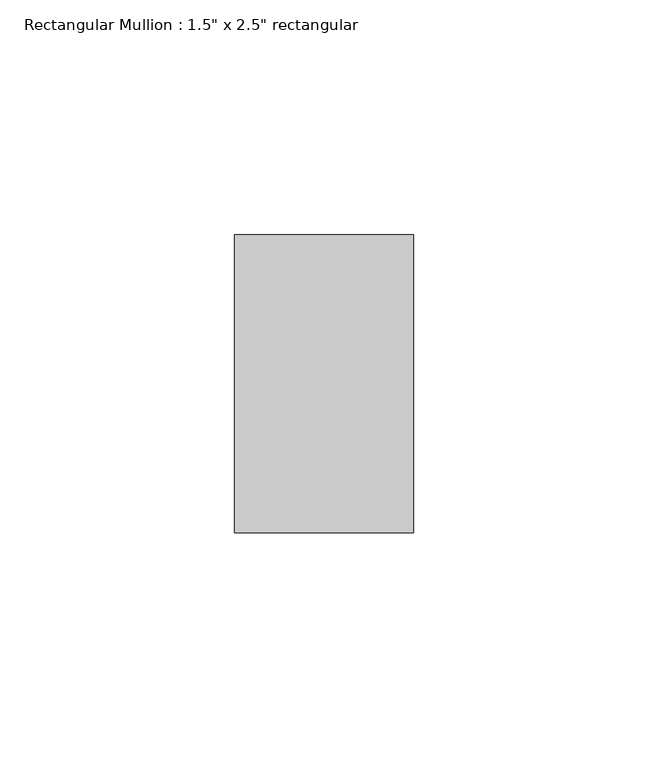
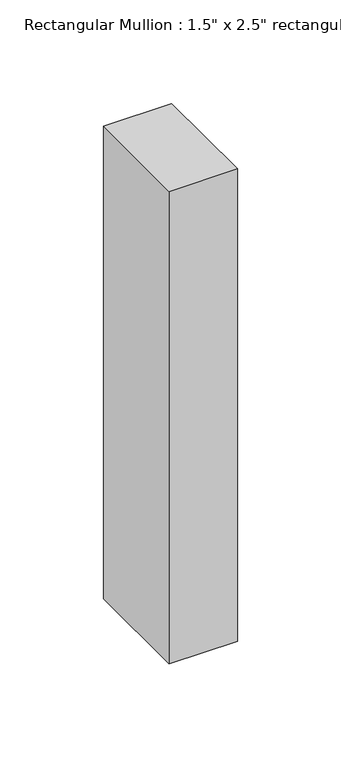
"""IFC4 building model written with IfcOpenShell, lengths in millimetres: member geometry."""

from ifc_helpers import new_model, si_unit, frame, origin, place, context, project, spatial, polyline, outline, extrude, source, transform, mapped, element, save


def member_5e1cd3ea(model_context):
    return source(origin(), model_context, "Body", "SweptSolid", [
        extrude(outline(polyline([(0.0, 31.75), (0.0, -31.75), (-38.1, -31.75), (-38.1, 31.75), (0.0, 31.75)])), frame((0.0, 0.0, -278.5951523), z_axis=(0.0, 0.0, 1.0), x_axis=(1.0, 0.0, 0.0)), (0.0, 0.0, 1.0), 278.5951523),
    ])


if __name__ == "__main__":
    model = new_model("IFC4")
    model_context = context("Model", 3, world=origin())
    ifc_project = project(units=[si_unit("LENGTHUNIT", "METRE", prefix="MILLI")], contexts=[model_context])
    site = spatial("IfcSite", under=ifc_project)
    building = spatial("IfcBuilding", under=site)
    placement = place(None, origin())
    member_shape = member_5e1cd3ea(model_context)
    element("IfcMember", 1, ObjectType="Rectangular Mullion : 1.5\" x 2.5\" rectangular", at=placement, inside=building, context=model_context, shape_type="MappedRepresentation", body=[
        mapped(member_shape, transform((0.0, 0.0, 0.0), x_axis=(1.0, 0.0, 0.0), y_axis=(0.0, 1.0, 0.0), z_axis=(0.0, 0.0, 1.0))),
    ])
    save(model, "model.ifc")

# Revit data of these elements
# Type "Rectangular Mullion : 1.5\" x 2.5\" rectangular"
#   built-in parameter 1007304 = 0.208333 (stored number, unit not read)
#   built-in parameter 1007301 = 0.0625 (stored number, unit not read)
#   built-in parameter 1007300 = 0.0625 (stored number, unit not read)
# Element 1 (IfcMember, "Rectangular Mullion : 1.5\" x 2.5\" rectangular")
#   Materials on its faces: "Leather - Black"
# Materials
#   "Leather - Black": class "Generic", colour RGB 40 40 40, transparency 0, Cost = 0
